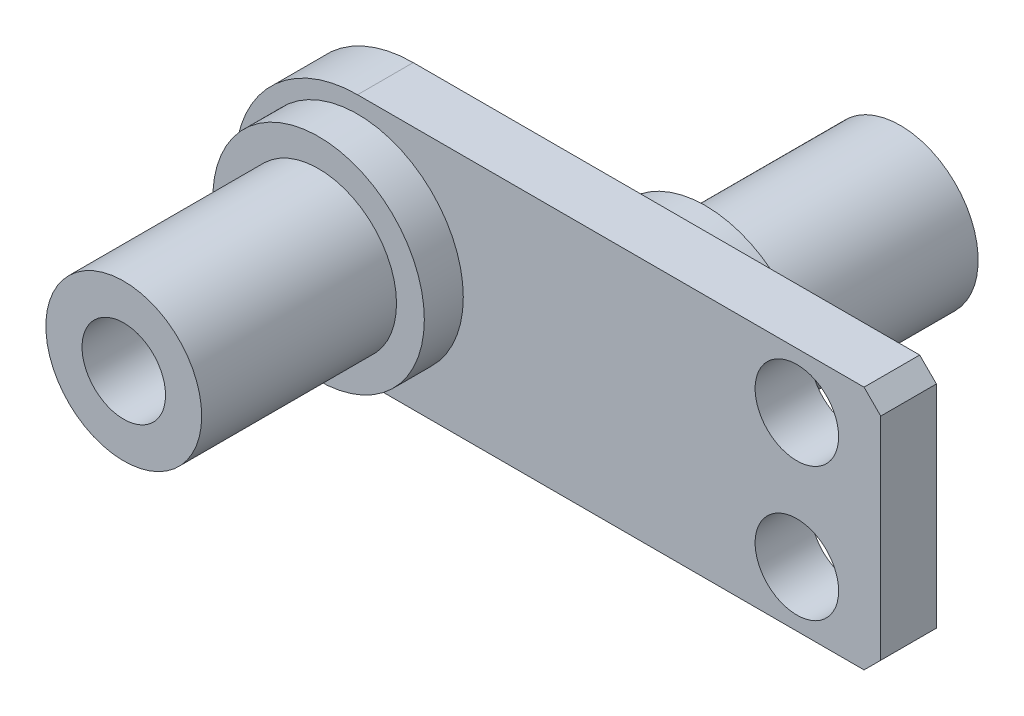
ISO-10303-21;
HEADER;
FILE_DESCRIPTION(('STEP AP214'),'2;1');
FILE_NAME('part.step','',(''),(''),'','','');
FILE_SCHEMA(('AUTOMOTIVE_DESIGN { 1 0 10303 214 1 1 1 1 }'));
ENDSEC;
DATA;
#1=APPLICATION_CONTEXT('core data for automotive mechanical design processes');
#2=APPLICATION_PROTOCOL_DEFINITION('international standard','automotive_design',2000,#1);
#3=PRODUCT_CONTEXT('',#1,'mechanical');
#4=PRODUCT('Part','Part','',(#3));
#5=PRODUCT_RELATED_PRODUCT_CATEGORY('part','',(#4));
#6=PRODUCT_DEFINITION_FORMATION('','',#4);
#7=PRODUCT_DEFINITION_CONTEXT('part definition',#1,'design');
#8=PRODUCT_DEFINITION('design','',#6,#7);
#9=PRODUCT_DEFINITION_SHAPE('','',#8);
#10=(LENGTH_UNIT() NAMED_UNIT(*) SI_UNIT(.MILLI.,.METRE.));
#11=(NAMED_UNIT(*) PLANE_ANGLE_UNIT() SI_UNIT($,.RADIAN.));
#12=(NAMED_UNIT(*) SI_UNIT($,.STERADIAN.) SOLID_ANGLE_UNIT());
#13=UNCERTAINTY_MEASURE_WITH_UNIT(LENGTH_MEASURE(1.E-05),#10,'distance_accuracy_value','');
#14=(GEOMETRIC_REPRESENTATION_CONTEXT(3) GLOBAL_UNCERTAINTY_ASSIGNED_CONTEXT((#13)) GLOBAL_UNIT_ASSIGNED_CONTEXT((#10,
#11,#12)) REPRESENTATION_CONTEXT('',''));
#15=CARTESIAN_POINT('',(0.,0.,0.));
#16=DIRECTION('',(0.,0.,1.));
#17=DIRECTION('',(1.,0.,0.));
#18=AXIS2_PLACEMENT_3D('',#15,#16,#17);
#19=CARTESIAN_POINT('',(0.,0.,10.));
#20=DIRECTION('',(0.,0.,-1.));
#21=DIRECTION('',(-1.,0.,0.));
#22=AXIS2_PLACEMENT_3D('',#19,#20,#21);
#23=CYLINDRICAL_SURFACE('',#22,22.);
#24=CARTESIAN_POINT('',(0.,0.,0.));
#25=DIRECTION('',(0.,0.,1.));
#26=DIRECTION('',(1.,0.,0.));
#27=AXIS2_PLACEMENT_3D('',#24,#25,#26);
#28=CIRCLE('',#27,22.);
#29=CARTESIAN_POINT('',(0.,22.,0.));
#30=VERTEX_POINT('',#29);
#31=CARTESIAN_POINT('',(0.,-22.,0.));
#32=VERTEX_POINT('',#31);
#33=EDGE_CURVE('E128',#30,#32,#28,.T.);
#34=ORIENTED_EDGE('',*,*,#33,.T.);
#35=DIRECTION('',(0.,0.,-1.));
#36=VECTOR('',#35,1.);
#37=CARTESIAN_POINT('',(0.,-22.,10.));
#38=LINE('',#37,#36);
#39=CARTESIAN_POINT('',(0.,-22.,10.));
#40=VERTEX_POINT('',#39);
#41=EDGE_CURVE('E149',#40,#32,#38,.T.);
#42=ORIENTED_EDGE('',*,*,#41,.F.);
#43=CARTESIAN_POINT('',(0.,0.,10.));
#44=DIRECTION('',(0.,0.,1.));
#45=DIRECTION('',(1.,0.,0.));
#46=AXIS2_PLACEMENT_3D('',#43,#44,#45);
#47=CIRCLE('',#46,22.);
#48=CARTESIAN_POINT('',(0.,22.,10.));
#49=VERTEX_POINT('',#48);
#50=EDGE_CURVE('E145',#49,#40,#47,.T.);
#51=ORIENTED_EDGE('',*,*,#50,.F.);
#52=DIRECTION('',(0.,0.,-1.));
#53=VECTOR('',#52,1.);
#54=CARTESIAN_POINT('',(0.,22.,10.));
#55=LINE('',#54,#53);
#56=EDGE_CURVE('E127',#49,#30,#55,.T.);
#57=ORIENTED_EDGE('',*,*,#56,.T.);
#58=EDGE_LOOP('',(#34,#42,#51,#57));
#59=FACE_BOUND('',#58,.T.);
#60=ADVANCED_FACE('F43',(#59),#23,.T.);
#61=CARTESIAN_POINT('',(69.,-22.,10.));
#62=DIRECTION('',(0.,1.,0.));
#63=DIRECTION('',(0.,0.,1.));
#64=AXIS2_PLACEMENT_3D('',#61,#62,#63);
#65=PLANE('',#64);
#66=DIRECTION('',(1.,0.,0.));
#67=VECTOR('',#66,1.);
#68=CARTESIAN_POINT('',(69.,-22.,0.));
#69=LINE('',#68,#67);
#70=CARTESIAN_POINT('',(91.,-22.,0.));
#71=VERTEX_POINT('',#70);
#72=EDGE_CURVE('E131',#32,#71,#69,.T.);
#73=ORIENTED_EDGE('',*,*,#72,.T.);
#74=DIRECTION('',(0.,0.,-1.));
#75=VECTOR('',#74,1.);
#76=CARTESIAN_POINT('',(91.,-22.,10.));
#77=LINE('',#76,#75);
#78=CARTESIAN_POINT('',(91.,-22.,10.));
#79=VERTEX_POINT('',#78);
#80=EDGE_CURVE('E147',#79,#71,#77,.T.);
#81=ORIENTED_EDGE('',*,*,#80,.F.);
#82=DIRECTION('',(1.,0.,0.));
#83=VECTOR('',#82,1.);
#84=CARTESIAN_POINT('',(0.,-22.,10.));
#85=LINE('',#84,#83);
#86=EDGE_CURVE('E98',#40,#79,#85,.T.);
#87=ORIENTED_EDGE('',*,*,#86,.F.);
#88=ORIENTED_EDGE('',*,*,#41,.T.);
#89=EDGE_LOOP('',(#73,#81,#87,#88));
#90=FACE_BOUND('',#89,.T.);
#91=ADVANCED_FACE('F170',(#90),#65,.F.);
#92=CARTESIAN_POINT('',(91.,-22.,10.));
#93=DIRECTION('',(-0.707106781186547,0.707106781186548,0.));
#94=DIRECTION('',(-0.707106781186548,-0.707106781186547,0.));
#95=AXIS2_PLACEMENT_3D('',#92,#93,#94);
#96=PLANE('',#95);
#97=DIRECTION('',(0.707106781186548,0.707106781186547,0.));
#98=VECTOR('',#97,1.);
#99=CARTESIAN_POINT('',(91.,-22.,0.));
#100=LINE('',#99,#98);
#101=CARTESIAN_POINT('',(94.,-19.,0.));
#102=VERTEX_POINT('',#101);
#103=EDGE_CURVE('E136',#71,#102,#100,.T.);
#104=ORIENTED_EDGE('',*,*,#103,.T.);
#105=DIRECTION('',(0.,0.,-1.));
#106=VECTOR('',#105,1.);
#107=CARTESIAN_POINT('',(94.,-19.,10.));
#108=LINE('',#107,#106);
#109=CARTESIAN_POINT('',(94.,-19.,10.));
#110=VERTEX_POINT('',#109);
#111=EDGE_CURVE('E122',#110,#102,#108,.T.);
#112=ORIENTED_EDGE('',*,*,#111,.F.);
#113=DIRECTION('',(0.707106781186548,0.707106781186547,0.));
#114=VECTOR('',#113,1.);
#115=CARTESIAN_POINT('',(91.,-22.,10.));
#116=LINE('',#115,#114);
#117=EDGE_CURVE('E109',#79,#110,#116,.T.);
#118=ORIENTED_EDGE('',*,*,#117,.F.);
#119=ORIENTED_EDGE('',*,*,#80,.T.);
#120=EDGE_LOOP('',(#104,#112,#118,#119));
#121=FACE_BOUND('',#120,.T.);
#122=ADVANCED_FACE('F167',(#121),#96,.F.);
#123=CARTESIAN_POINT('',(94.,19.,10.));
#124=DIRECTION('',(-1.,0.,0.));
#125=DIRECTION('',(0.,0.,1.));
#126=AXIS2_PLACEMENT_3D('',#123,#124,#125);
#127=PLANE('',#126);
#128=DIRECTION('',(0.,1.,0.));
#129=VECTOR('',#128,1.);
#130=CARTESIAN_POINT('',(94.,19.,0.));
#131=LINE('',#130,#129);
#132=CARTESIAN_POINT('',(94.,19.,0.));
#133=VERTEX_POINT('',#132);
#134=EDGE_CURVE('E118',#102,#133,#131,.T.);
#135=ORIENTED_EDGE('',*,*,#134,.T.);
#136=DIRECTION('',(0.,0.,-1.));
#137=VECTOR('',#136,1.);
#138=CARTESIAN_POINT('',(94.,19.,10.));
#139=LINE('',#138,#137);
#140=CARTESIAN_POINT('',(94.,19.,10.));
#141=VERTEX_POINT('',#140);
#142=EDGE_CURVE('E116',#141,#133,#139,.T.);
#143=ORIENTED_EDGE('',*,*,#142,.F.);
#144=DIRECTION('',(0.,1.,0.));
#145=VECTOR('',#144,1.);
#146=CARTESIAN_POINT('',(94.,19.,10.));
#147=LINE('',#146,#145);
#148=EDGE_CURVE('E101',#110,#141,#147,.T.);
#149=ORIENTED_EDGE('',*,*,#148,.F.);
#150=ORIENTED_EDGE('',*,*,#111,.T.);
#151=EDGE_LOOP('',(#135,#143,#149,#150));
#152=FACE_BOUND('',#151,.T.);
#153=ADVANCED_FACE('F120',(#152),#127,.F.);
#154=CARTESIAN_POINT('',(91.,22.,10.));
#155=DIRECTION('',(-0.707106781186547,-0.707106781186548,0.));
#156=DIRECTION('',(0.707106781186548,-0.707106781186547,0.));
#157=AXIS2_PLACEMENT_3D('',#154,#155,#156);
#158=PLANE('',#157);
#159=DIRECTION('',(-0.707106781186548,0.707106781186547,0.));
#160=VECTOR('',#159,1.);
#161=CARTESIAN_POINT('',(91.,22.,0.));
#162=LINE('',#161,#160);
#163=CARTESIAN_POINT('',(91.,22.,0.));
#164=VERTEX_POINT('',#163);
#165=EDGE_CURVE('E137',#133,#164,#162,.T.);
#166=ORIENTED_EDGE('',*,*,#165,.T.);
#167=DIRECTION('',(0.,0.,-1.));
#168=VECTOR('',#167,1.);
#169=CARTESIAN_POINT('',(91.,22.,10.));
#170=LINE('',#169,#168);
#171=CARTESIAN_POINT('',(91.,22.,10.));
#172=VERTEX_POINT('',#171);
#173=EDGE_CURVE('E125',#172,#164,#170,.T.);
#174=ORIENTED_EDGE('',*,*,#173,.F.);
#175=DIRECTION('',(-0.707106781186548,0.707106781186547,0.));
#176=VECTOR('',#175,1.);
#177=CARTESIAN_POINT('',(91.,22.,10.));
#178=LINE('',#177,#176);
#179=EDGE_CURVE('E110',#141,#172,#178,.T.);
#180=ORIENTED_EDGE('',*,*,#179,.F.);
#181=ORIENTED_EDGE('',*,*,#142,.T.);
#182=EDGE_LOOP('',(#166,#174,#180,#181));
#183=FACE_BOUND('',#182,.T.);
#184=ADVANCED_FACE('F121',(#183),#158,.F.);
#185=CARTESIAN_POINT('',(0.,22.,10.));
#186=DIRECTION('',(0.,-1.,0.));
#187=DIRECTION('',(0.,0.,-1.));
#188=AXIS2_PLACEMENT_3D('',#185,#186,#187);
#189=PLANE('',#188);
#190=DIRECTION('',(-1.,0.,0.));
#191=VECTOR('',#190,1.);
#192=CARTESIAN_POINT('',(0.,22.,0.));
#193=LINE('',#192,#191);
#194=EDGE_CURVE('E84',#164,#30,#193,.T.);
#195=ORIENTED_EDGE('',*,*,#194,.T.);
#196=ORIENTED_EDGE('',*,*,#56,.F.);
#197=DIRECTION('',(-1.,0.,0.));
#198=VECTOR('',#197,1.);
#199=CARTESIAN_POINT('',(69.,22.,10.));
#200=LINE('',#199,#198);
#201=EDGE_CURVE('E58',#172,#49,#200,.T.);
#202=ORIENTED_EDGE('',*,*,#201,.F.);
#203=ORIENTED_EDGE('',*,*,#173,.T.);
#204=EDGE_LOOP('',(#195,#196,#202,#203));
#205=FACE_BOUND('',#204,.T.);
#206=ADVANCED_FACE('F175',(#205),#189,.F.);
#207=CARTESIAN_POINT('',(0.,0.,10.));
#208=DIRECTION('',(0.,0.,1.));
#209=DIRECTION('',(1.,0.,0.));
#210=AXIS2_PLACEMENT_3D('',#207,#208,#209);
#211=PLANE('',#210);
#212=CARTESIAN_POINT('',(78.9291881107862,12.,10.));
#213=DIRECTION('',(0.,0.,1.));
#214=DIRECTION('',(1.,0.,0.));
#215=AXIS2_PLACEMENT_3D('',#212,#213,#214);
#216=CIRCLE('',#215,7.5);
#217=CARTESIAN_POINT('',(86.4291881107862,12.,10.));
#218=VERTEX_POINT('',#217);
#219=EDGE_CURVE('E259',#218,#218,#216,.T.);
#220=ORIENTED_EDGE('',*,*,#219,.F.);
#221=EDGE_LOOP('',(#220));
#222=FACE_BOUND('',#221,.T.);
#223=CARTESIAN_POINT('',(78.9291881107862,-12.,10.));
#224=DIRECTION('',(0.,0.,1.));
#225=DIRECTION('',(1.,0.,0.));
#226=AXIS2_PLACEMENT_3D('',#223,#224,#225);
#227=CIRCLE('',#226,7.50000000000001);
#228=CARTESIAN_POINT('',(86.4291881107862,-12.,10.));
#229=VERTEX_POINT('',#228);
#230=EDGE_CURVE('E262',#229,#229,#227,.T.);
#231=ORIENTED_EDGE('',*,*,#230,.F.);
#232=EDGE_LOOP('',(#231));
#233=FACE_BOUND('',#232,.T.);
#234=CARTESIAN_POINT('',(0.,0.,10.));
#235=DIRECTION('',(0.,0.,1.));
#236=DIRECTION('',(1.,0.,0.));
#237=AXIS2_PLACEMENT_3D('',#234,#235,#236);
#238=CIRCLE('',#237,19.);
#239=CARTESIAN_POINT('',(19.,0.,10.));
#240=VERTEX_POINT('',#239);
#241=EDGE_CURVE('E162',#240,#240,#238,.T.);
#242=ORIENTED_EDGE('',*,*,#241,.F.);
#243=EDGE_LOOP('',(#242));
#244=FACE_BOUND('',#243,.T.);
#245=ORIENTED_EDGE('',*,*,#50,.T.);
#246=ORIENTED_EDGE('',*,*,#86,.T.);
#247=ORIENTED_EDGE('',*,*,#117,.T.);
#248=ORIENTED_EDGE('',*,*,#148,.T.);
#249=ORIENTED_EDGE('',*,*,#179,.T.);
#250=ORIENTED_EDGE('',*,*,#201,.T.);
#251=EDGE_LOOP('',(#245,#246,#247,#248,#249,#250));
#252=FACE_BOUND('',#251,.T.);
#253=ADVANCED_FACE('F102',(#222,#233,#244,#252),#211,.T.);
#254=CARTESIAN_POINT('',(0.,0.,0.));
#255=DIRECTION('',(0.,0.,1.));
#256=DIRECTION('',(1.,0.,0.));
#257=AXIS2_PLACEMENT_3D('',#254,#255,#256);
#258=PLANE('',#257);
#259=CARTESIAN_POINT('',(78.9291881107862,12.,0.));
#260=DIRECTION('',(0.,0.,1.));
#261=DIRECTION('',(1.,0.,0.));
#262=AXIS2_PLACEMENT_3D('',#259,#260,#261);
#263=CIRCLE('',#262,7.5);
#264=CARTESIAN_POINT('',(86.4291881107862,12.,0.));
#265=VERTEX_POINT('',#264);
#266=EDGE_CURVE('E253',#265,#265,#263,.T.);
#267=ORIENTED_EDGE('',*,*,#266,.T.);
#268=EDGE_LOOP('',(#267));
#269=FACE_BOUND('',#268,.T.);
#270=CARTESIAN_POINT('',(78.9291881107862,-12.,0.));
#271=DIRECTION('',(0.,0.,1.));
#272=DIRECTION('',(1.,0.,0.));
#273=AXIS2_PLACEMENT_3D('',#270,#271,#272);
#274=CIRCLE('',#273,7.50000000000001);
#275=CARTESIAN_POINT('',(86.4291881107862,-12.,0.));
#276=VERTEX_POINT('',#275);
#277=EDGE_CURVE('E256',#276,#276,#274,.T.);
#278=ORIENTED_EDGE('',*,*,#277,.T.);
#279=EDGE_LOOP('',(#278));
#280=FACE_BOUND('',#279,.T.);
#281=CARTESIAN_POINT('',(45.5,0.,0.));
#282=DIRECTION('',(0.,0.,1.));
#283=DIRECTION('',(1.,0.,0.));
#284=AXIS2_PLACEMENT_3D('',#281,#282,#283);
#285=CIRCLE('',#284,19.);
#286=CARTESIAN_POINT('',(64.5,0.,0.));
#287=VERTEX_POINT('',#286);
#288=EDGE_CURVE('E46',#287,#287,#285,.F.);
#289=ORIENTED_EDGE('',*,*,#288,.F.);
#290=EDGE_LOOP('',(#289));
#291=FACE_BOUND('',#290,.T.);
#292=ORIENTED_EDGE('',*,*,#33,.F.);
#293=ORIENTED_EDGE('',*,*,#194,.F.);
#294=ORIENTED_EDGE('',*,*,#165,.F.);
#295=ORIENTED_EDGE('',*,*,#134,.F.);
#296=ORIENTED_EDGE('',*,*,#103,.F.);
#297=ORIENTED_EDGE('',*,*,#72,.F.);
#298=EDGE_LOOP('',(#292,#293,#294,#295,#296,#297));
#299=FACE_BOUND('',#298,.T.);
#300=ADVANCED_FACE('F171',(#269,#280,#291,#299),#258,.F.);
#301=CARTESIAN_POINT('',(0.,0.,17.));
#302=DIRECTION('',(0.,0.,-1.));
#303=DIRECTION('',(-1.,0.,0.));
#304=AXIS2_PLACEMENT_3D('',#301,#302,#303);
#305=CYLINDRICAL_SURFACE('',#304,19.);
#306=CARTESIAN_POINT('',(0.,0.,17.));
#307=DIRECTION('',(0.,0.,1.));
#308=DIRECTION('',(1.,0.,0.));
#309=AXIS2_PLACEMENT_3D('',#306,#307,#308);
#310=CIRCLE('',#309,19.);
#311=CARTESIAN_POINT('',(19.,0.,17.));
#312=VERTEX_POINT('',#311);
#313=EDGE_CURVE('E132',#312,#312,#310,.T.);
#314=ORIENTED_EDGE('',*,*,#313,.F.);
#315=EDGE_LOOP('',(#314));
#316=FACE_BOUND('',#315,.T.);
#317=ORIENTED_EDGE('',*,*,#241,.T.);
#318=EDGE_LOOP('',(#317));
#319=FACE_BOUND('',#318,.T.);
#320=ADVANCED_FACE('F192',(#316,#319),#305,.T.);
#321=CARTESIAN_POINT('',(0.,0.,17.));
#322=DIRECTION('',(0.,0.,1.));
#323=DIRECTION('',(1.,0.,0.));
#324=AXIS2_PLACEMENT_3D('',#321,#322,#323);
#325=PLANE('',#324);
#326=CARTESIAN_POINT('',(0.,0.,17.));
#327=DIRECTION('',(0.,0.,1.));
#328=DIRECTION('',(1.,0.,0.));
#329=AXIS2_PLACEMENT_3D('',#326,#327,#328);
#330=CIRCLE('',#329,14.);
#331=CARTESIAN_POINT('',(14.,0.,17.));
#332=VERTEX_POINT('',#331);
#333=EDGE_CURVE('E146',#332,#332,#330,.T.);
#334=ORIENTED_EDGE('',*,*,#333,.F.);
#335=EDGE_LOOP('',(#334));
#336=FACE_BOUND('',#335,.T.);
#337=ORIENTED_EDGE('',*,*,#313,.T.);
#338=EDGE_LOOP('',(#337));
#339=FACE_BOUND('',#338,.T.);
#340=ADVANCED_FACE('F196',(#336,#339),#325,.T.);
#341=CARTESIAN_POINT('',(0.,0.,52.));
#342=DIRECTION('',(0.,0.,-1.));
#343=DIRECTION('',(-1.,0.,0.));
#344=AXIS2_PLACEMENT_3D('',#341,#342,#343);
#345=CYLINDRICAL_SURFACE('',#344,14.);
#346=CARTESIAN_POINT('',(0.,0.,52.));
#347=DIRECTION('',(0.,0.,1.));
#348=DIRECTION('',(1.,0.,0.));
#349=AXIS2_PLACEMENT_3D('',#346,#347,#348);
#350=CIRCLE('',#349,14.);
#351=CARTESIAN_POINT('',(14.,0.,52.));
#352=VERTEX_POINT('',#351);
#353=EDGE_CURVE('E158',#352,#352,#350,.T.);
#354=ORIENTED_EDGE('',*,*,#353,.F.);
#355=EDGE_LOOP('',(#354));
#356=FACE_BOUND('',#355,.T.);
#357=ORIENTED_EDGE('',*,*,#333,.T.);
#358=EDGE_LOOP('',(#357));
#359=FACE_BOUND('',#358,.T.);
#360=ADVANCED_FACE('F205',(#356,#359),#345,.T.);
#361=CARTESIAN_POINT('',(0.,0.,52.));
#362=DIRECTION('',(0.,0.,1.));
#363=DIRECTION('',(1.,0.,0.));
#364=AXIS2_PLACEMENT_3D('',#361,#362,#363);
#365=PLANE('',#364);
#366=CARTESIAN_POINT('',(0.,0.,52.));
#367=DIRECTION('',(0.,0.,1.));
#368=DIRECTION('',(1.,0.,0.));
#369=AXIS2_PLACEMENT_3D('',#366,#367,#368);
#370=CIRCLE('',#369,7.5);
#371=CARTESIAN_POINT('',(7.5,0.,52.));
#372=VERTEX_POINT('',#371);
#373=EDGE_CURVE('E263',#372,#372,#370,.T.);
#374=ORIENTED_EDGE('',*,*,#373,.F.);
#375=EDGE_LOOP('',(#374));
#376=FACE_BOUND('',#375,.T.);
#377=ORIENTED_EDGE('',*,*,#353,.T.);
#378=EDGE_LOOP('',(#377));
#379=FACE_BOUND('',#378,.T.);
#380=ADVANCED_FACE('F207',(#376,#379),#365,.T.);
#381=CARTESIAN_POINT('',(45.5,0.,-7.));
#382=DIRECTION('',(0.,0.,1.));
#383=DIRECTION('',(1.,0.,0.));
#384=AXIS2_PLACEMENT_3D('',#381,#382,#383);
#385=CYLINDRICAL_SURFACE('',#384,19.);
#386=CARTESIAN_POINT('',(45.5,0.,-7.));
#387=DIRECTION('',(0.,0.,-1.));
#388=DIRECTION('',(-1.,0.,0.));
#389=AXIS2_PLACEMENT_3D('',#386,#387,#388);
#390=CIRCLE('',#389,19.);
#391=CARTESIAN_POINT('',(26.5,0.,-7.));
#392=VERTEX_POINT('',#391);
#393=EDGE_CURVE('E285',#392,#392,#390,.T.);
#394=ORIENTED_EDGE('',*,*,#393,.F.);
#395=EDGE_LOOP('',(#394));
#396=FACE_BOUND('',#395,.T.);
#397=ORIENTED_EDGE('',*,*,#288,.T.);
#398=EDGE_LOOP('',(#397));
#399=FACE_BOUND('',#398,.T.);
#400=ADVANCED_FACE('F208',(#396,#399),#385,.T.);
#401=CARTESIAN_POINT('',(45.5,0.,-7.));
#402=DIRECTION('',(0.,0.,-1.));
#403=DIRECTION('',(-1.,0.,0.));
#404=AXIS2_PLACEMENT_3D('',#401,#402,#403);
#405=PLANE('',#404);
#406=CARTESIAN_POINT('',(45.5,0.,-7.));
#407=DIRECTION('',(0.,0.,-1.));
#408=DIRECTION('',(-1.,0.,0.));
#409=AXIS2_PLACEMENT_3D('',#406,#407,#408);
#410=CIRCLE('',#409,14.);
#411=CARTESIAN_POINT('',(31.5,0.,-7.));
#412=VERTEX_POINT('',#411);
#413=EDGE_CURVE('E11',#412,#412,#410,.T.);
#414=ORIENTED_EDGE('',*,*,#413,.F.);
#415=EDGE_LOOP('',(#414));
#416=FACE_BOUND('',#415,.T.);
#417=ORIENTED_EDGE('',*,*,#393,.T.);
#418=EDGE_LOOP('',(#417));
#419=FACE_BOUND('',#418,.T.);
#420=ADVANCED_FACE('F211',(#416,#419),#405,.T.);
#421=CARTESIAN_POINT('',(45.5,0.,-42.));
#422=DIRECTION('',(0.,0.,1.));
#423=DIRECTION('',(1.,0.,0.));
#424=AXIS2_PLACEMENT_3D('',#421,#422,#423);
#425=CYLINDRICAL_SURFACE('',#424,14.);
#426=CARTESIAN_POINT('',(45.5,0.,-42.));
#427=DIRECTION('',(0.,0.,-1.));
#428=DIRECTION('',(-1.,0.,0.));
#429=AXIS2_PLACEMENT_3D('',#426,#427,#428);
#430=CIRCLE('',#429,14.);
#431=CARTESIAN_POINT('',(31.5,0.,-42.));
#432=VERTEX_POINT('',#431);
#433=EDGE_CURVE('E279',#432,#432,#430,.T.);
#434=ORIENTED_EDGE('',*,*,#433,.F.);
#435=EDGE_LOOP('',(#434));
#436=FACE_BOUND('',#435,.T.);
#437=ORIENTED_EDGE('',*,*,#413,.T.);
#438=EDGE_LOOP('',(#437));
#439=FACE_BOUND('',#438,.T.);
#440=ADVANCED_FACE('F216',(#436,#439),#425,.T.);
#441=CARTESIAN_POINT('',(45.5,0.,-42.));
#442=DIRECTION('',(0.,0.,-1.));
#443=DIRECTION('',(-1.,0.,0.));
#444=AXIS2_PLACEMENT_3D('',#441,#442,#443);
#445=PLANE('',#444);
#446=CARTESIAN_POINT('',(45.5,0.,-42.));
#447=DIRECTION('',(0.,0.,-1.));
#448=DIRECTION('',(-1.,0.,0.));
#449=AXIS2_PLACEMENT_3D('',#446,#447,#448);
#450=CIRCLE('',#449,7.5);
#451=CARTESIAN_POINT('',(38.,0.,-42.));
#452=VERTEX_POINT('',#451);
#453=EDGE_CURVE('E275',#452,#452,#450,.T.);
#454=ORIENTED_EDGE('',*,*,#453,.F.);
#455=EDGE_LOOP('',(#454));
#456=FACE_BOUND('',#455,.T.);
#457=ORIENTED_EDGE('',*,*,#433,.T.);
#458=EDGE_LOOP('',(#457));
#459=FACE_BOUND('',#458,.T.);
#460=ADVANCED_FACE('F225',(#456,#459),#445,.T.);
#461=CARTESIAN_POINT('',(45.5,0.,-7.));
#462=DIRECTION('',(0.,0.,-1.));
#463=DIRECTION('',(-1.,0.,0.));
#464=AXIS2_PLACEMENT_3D('',#461,#462,#463);
#465=CYLINDRICAL_SURFACE('',#464,7.5);
#466=CARTESIAN_POINT('',(45.5,0.,-7.));
#467=DIRECTION('',(0.,0.,-1.));
#468=DIRECTION('',(-1.,0.,0.));
#469=AXIS2_PLACEMENT_3D('',#466,#467,#468);
#470=CIRCLE('',#469,7.5);
#471=CARTESIAN_POINT('',(38.,0.,-7.));
#472=VERTEX_POINT('',#471);
#473=EDGE_CURVE('E273',#472,#472,#470,.T.);
#474=ORIENTED_EDGE('',*,*,#473,.F.);
#475=EDGE_LOOP('',(#474));
#476=FACE_BOUND('',#475,.T.);
#477=ORIENTED_EDGE('',*,*,#453,.T.);
#478=EDGE_LOOP('',(#477));
#479=FACE_BOUND('',#478,.T.);
#480=ADVANCED_FACE('F228',(#476,#479),#465,.F.);
#481=CARTESIAN_POINT('',(45.5,0.,-7.));
#482=DIRECTION('',(0.,0.,-1.));
#483=DIRECTION('',(-1.,0.,0.));
#484=AXIS2_PLACEMENT_3D('',#481,#482,#483);
#485=PLANE('',#484);
#486=ORIENTED_EDGE('',*,*,#473,.T.);
#487=EDGE_LOOP('',(#486));
#488=FACE_BOUND('',#487,.T.);
#489=ADVANCED_FACE('F229',(#488),#485,.T.);
#490=CARTESIAN_POINT('',(0.,0.,17.));
#491=DIRECTION('',(0.,0.,1.));
#492=DIRECTION('',(1.,0.,0.));
#493=AXIS2_PLACEMENT_3D('',#490,#491,#492);
#494=CYLINDRICAL_SURFACE('',#493,7.5);
#495=CARTESIAN_POINT('',(0.,0.,17.));
#496=DIRECTION('',(0.,0.,1.));
#497=DIRECTION('',(1.,0.,0.));
#498=AXIS2_PLACEMENT_3D('',#495,#496,#497);
#499=CIRCLE('',#498,7.5);
#500=CARTESIAN_POINT('',(7.5,0.,17.));
#501=VERTEX_POINT('',#500);
#502=EDGE_CURVE('E267',#501,#501,#499,.T.);
#503=ORIENTED_EDGE('',*,*,#502,.F.);
#504=EDGE_LOOP('',(#503));
#505=FACE_BOUND('',#504,.T.);
#506=ORIENTED_EDGE('',*,*,#373,.T.);
#507=EDGE_LOOP('',(#506));
#508=FACE_BOUND('',#507,.T.);
#509=ADVANCED_FACE('F234',(#505,#508),#494,.F.);
#510=CARTESIAN_POINT('',(0.,0.,17.));
#511=DIRECTION('',(0.,0.,1.));
#512=DIRECTION('',(1.,0.,0.));
#513=AXIS2_PLACEMENT_3D('',#510,#511,#512);
#514=PLANE('',#513);
#515=ORIENTED_EDGE('',*,*,#502,.T.);
#516=EDGE_LOOP('',(#515));
#517=FACE_BOUND('',#516,.T.);
#518=ADVANCED_FACE('F238',(#517),#514,.T.);
#519=CARTESIAN_POINT('',(78.9291881107862,-12.,0.));
#520=DIRECTION('',(0.,0.,1.));
#521=DIRECTION('',(1.,0.,0.));
#522=AXIS2_PLACEMENT_3D('',#519,#520,#521);
#523=CYLINDRICAL_SURFACE('',#522,7.50000000000001);
#524=ORIENTED_EDGE('',*,*,#277,.F.);
#525=EDGE_LOOP('',(#524));
#526=FACE_BOUND('',#525,.T.);
#527=ORIENTED_EDGE('',*,*,#230,.T.);
#528=EDGE_LOOP('',(#527));
#529=FACE_BOUND('',#528,.T.);
#530=ADVANCED_FACE('F245',(#526,#529),#523,.F.);
#531=CARTESIAN_POINT('',(78.9291881107862,12.,0.));
#532=DIRECTION('',(0.,0.,1.));
#533=DIRECTION('',(1.,0.,0.));
#534=AXIS2_PLACEMENT_3D('',#531,#532,#533);
#535=CYLINDRICAL_SURFACE('',#534,7.5);
#536=ORIENTED_EDGE('',*,*,#266,.F.);
#537=EDGE_LOOP('',(#536));
#538=FACE_BOUND('',#537,.T.);
#539=ORIENTED_EDGE('',*,*,#219,.T.);
#540=EDGE_LOOP('',(#539));
#541=FACE_BOUND('',#540,.T.);
#542=ADVANCED_FACE('F246',(#538,#541),#535,.F.);
#543=CLOSED_SHELL('',(#60,#91,#122,#153,#184,#206,#253,#300,#320,#340,#360,#380,#400,#420,#440,
#460,#480,#489,#509,#518,#530,#542));
#544=MANIFOLD_SOLID_BREP('B2',#543);
#545=ADVANCED_BREP_SHAPE_REPRESENTATION('',(#18,#544),#14);
#546=SHAPE_DEFINITION_REPRESENTATION(#9,#545);
ENDSEC;
END-ISO-10303-21;
